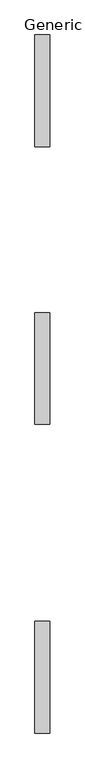
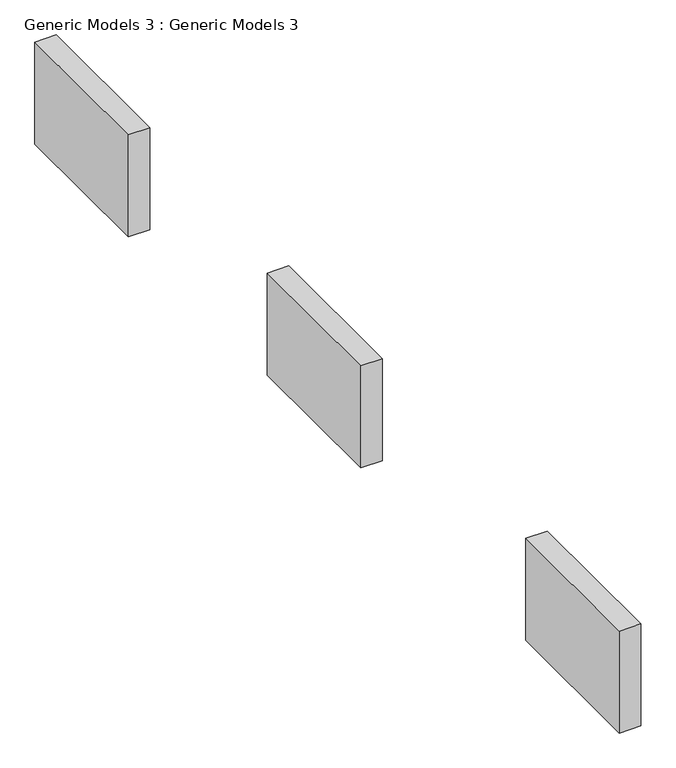
"""IFC4 building model written with IfcOpenShell, lengths in millimetres: proxy geometry, Generic Models 3 : Generic Models 3."""

from ifc_helpers import new_model, si_unit, frame, origin, place, context, project, spatial, polyline, outline, extrude, source, transform, mapped, element, save


def generic_models_3_generic_models_3_d2748d51(model_context):
    return source(origin(), model_context, "Body", "SweptSolid", [
        extrude(outline(polyline([(4476.1077953, -4753.4490872), (4476.1077953, -7039.4490872), (4171.3077953, -7039.4490872), (4171.3077953, -4753.4490872), (4476.1077953, -4753.4490872)])), frame((0.0, 0.0, 330.3723676), z_axis=(0.0, 0.0, 1.0), x_axis=(1.0, 0.0, 0.0)), (0.0, 0.0, 1.0), 1524.0),
        extrude(outline(polyline([(4476.1077953, 1571.1509128), (4476.1077953, -714.8490872), (4171.3077953, -714.8490872), (4171.3077953, 1571.1509128), (4476.1077953, 1571.1509128)])), frame((0.0, 0.0, 457.3723676), z_axis=(0.0, 0.0, 1.0), x_axis=(1.0, 0.0, 0.0)), (0.0, 0.0, 1.0), 1524.0),
        extrude(outline(polyline([(4476.1077953, 7260.7509128), (4476.1077953, 4974.7509128), (4171.3077953, 4974.7509128), (4171.3077953, 7260.7509128), (4476.1077953, 7260.7509128)])), frame((0.0, 0.0, 457.3723676), z_axis=(0.0, 0.0, 1.0), x_axis=(1.0, 0.0, 0.0)), (0.0, 0.0, 1.0), 1524.0),
    ])


if __name__ == "__main__":
    model = new_model("IFC4")
    model_context = context("Model", 3, world=origin())
    ifc_project = project(units=[si_unit("LENGTHUNIT", "METRE", prefix="MILLI")], contexts=[model_context])
    site = spatial("IfcSite", under=ifc_project)
    building = spatial("IfcBuilding", under=site)
    placement = place(None, origin())
    generic_models_3_generic_models_3_shape = generic_models_3_generic_models_3_d2748d51(model_context)
    element("IfcBuildingElementProxy", 1, Name="Generic Models 3 : Generic Models 3", ObjectType="Generic Models 3 : Generic Models 3", at=placement, inside=building, context=model_context, shape_type="MappedRepresentation", body=[
        mapped(generic_models_3_generic_models_3_shape, transform((0.0, 0.0, 0.0), x_axis=(1.0, 0.0, 0.0), y_axis=(0.0, 1.0, 0.0), z_axis=(0.0, 0.0, 1.0))),
    ])
    save(model, "model.ifc")

# Revit data of these elements
# Element 1 (IfcBuildingElementProxy, "Generic Models 3 : Generic Models 3")
#   Materials on its faces: "Parking Stripe"
# Materials
#   "Parking Stripe": class "Paint", colour RGB 250 250 91, transparency 0, Cost = 0
